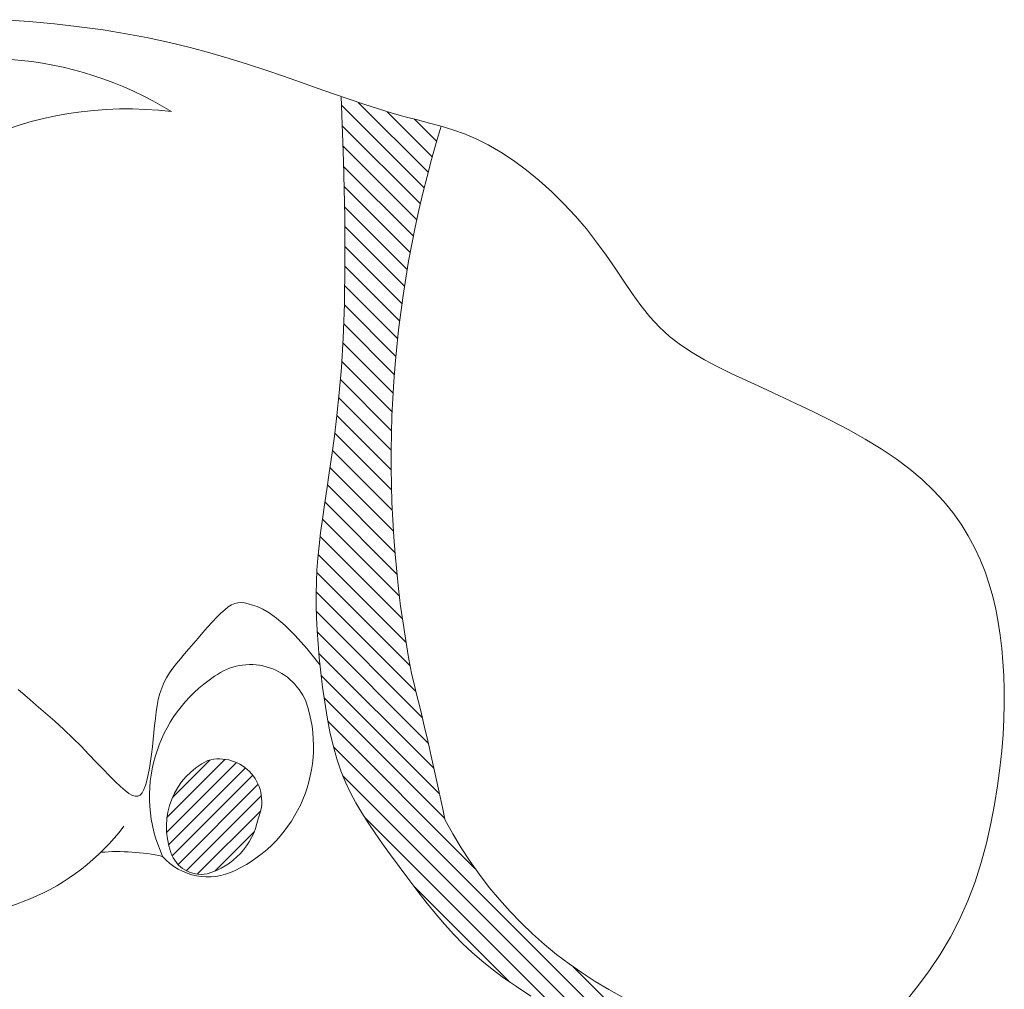
# Model space of a CAD drawing. Units: inches. Extents: x -17 to 1735, y -531 to 60.
# Tile 9 of 27: x 1734.675388 to 1734.678793, y -150.220021 to -150.216668. Entities that reach past the tile are written whole.
import ezdxf

# ---------------------------------------------------------------- set-up
doc = ezdxf.new("R2010")
doc.units = ezdxf.units.IN
doc.header["$MEASUREMENT"] = 0
doc.layers.add('A-FURN', color=242, linetype='Continuous', lineweight=18, true_color=0xcd2027)

# ---------------------------------------------------------------- blocks, each defined once
blk = doc.blocks.new('childrens_room_2')
for p, q in [((70.17339440191746, 54.15018009333147), (70.17563597329311, 54.15001020629865)), ((70.17563597329311, 54.15001020629865), (70.17785059184419, 54.14980570076153)), ((70.17785059184419, 54.14980570076153), (70.18001900573611, 54.14956273020511)), ((70.18001900573611, 54.14956273020511), (70.18212196290145, 54.14927744811433)), ((70.18212196290145, 54.14927744811433), (70.18414438255016, 54.14894745044733)), ((70.18414438255016, 54.14894745044733), (70.18608786917642, 54.14857610287294)), ((70.18608786917642, 54.14857610287294), (70.18795819820255, 54.14816821353309)), ((70.18795819820255, 54.14816821353309), (70.18976114540013, 54.14772859055523)), ((70.18976114540013, 54.14772859055523), (70.19150248619147, 54.14726204206676)), ((70.19150248619147, 54.14726204206676), (70.19318799628994, 54.14677337620964)), ((70.19318799628994, 54.14677337620964), (70.19482345123427, 54.14626740109674)), ((70.19482345123427, 54.14626740109674), (70.19641462662142, 54.14574892487729)), ((70.19641462662142, 54.14574892487729), (70.1979658542073, 54.14522323648128)), ((70.1979658542073, 54.14522323648128), (70.19947568997625, 54.14469754809255)), ((70.19947568997625, 54.14469754809255), (70.20094124624623, 54.14417955271932)), ((70.20094124624623, 54.14417955271932), (70.20235963521876, 54.14367694335528)), ((70.20235963521876, 54.14367694335528), (70.20372796909535, 54.14319741299408)), ((70.20304380218616, 54.14343717817832), (70.20324643027155, 54.13775630528693)), ((70.21032588458505, 54.13540639450224), (70.2030714949465, 54.14266078414079)), ((70.20372796909535, 54.14319741299408), (70.20504336001935, 54.14274865464398)), ((70.21067641210858, 54.13678467516587), (70.20454107237632, 54.14292001493453)), ((70.20504336001935, 54.14274865464398), (70.20630292025047, 54.14233836128409)), ((70.20630292025047, 54.14233836128409), (70.20750376199024, 54.14197422592991)), ((70.21104344307562, 54.13814645241513), (70.20709029149614, 54.14209960400916)), ((70.20750376199024, 54.14197422592991), (70.20864556439804, 54.14165913344771)), ((70.20864556439804, 54.14165913344771), (70.20973827429, 54.14137673621593)), ((70.21142657864723, 54.13949212503069), (70.20947355376441, 54.14144514992807)), ((70.20973827429, 54.14137673621593), (70.21079440544011, 54.14110587847102)), ((70.21079440544011, 54.14110587847102), (70.21182647162235, 54.14082540447856)), ((70.20999228646863, 54.13401118443147), (70.2031354397291, 54.14086803115646)), ((70.21182544513024, 54.14082206677125), (70.21182047879441, 54.14082703307798)), ((70.21182647162235, 54.14082540447856), (70.21284698661069, 54.14051415846774)), ((70.21284698661069, 54.14051415846774), (70.21386846423732, 54.14015098470412)), ((70.21386846423732, 54.14015098470412), (70.21490341821801, 54.13971472742417)), ((70.21490341821801, 54.13971472742417), (70.21596436232679, 54.1391842308862)), ((70.21596436232679, 54.1391842308862), (70.21705931827776, 54.13854378854598)), ((70.20967607329251, 54.13259858941313), (70.20319938451169, 54.13907527817213)), ((70.21705931827776, 54.13854378854598), (70.2181783391384, 54.13779949069288)), ((70.20324643027155, 54.13775630528693), (70.20335176733673, 54.13288732946097)), ((70.2181783391384, 54.13779949069288), (70.21930698597455, 54.13696287682836)), ((70.20937773283688, 54.13116812163792), (70.20325653320063, 54.13728932131784)), ((70.21930698597455, 54.13696287682836), (70.22043081979385, 54.13604548646111)), ((70.22043081979385, 54.13604548646111), (70.22153540166212, 54.13505885909256)), ((70.2090977882722, 54.1297192580518), (70.20329476183863, 54.13552228446355)), ((70.22153540166212, 54.13505885909256), (70.22260629252881, 54.13401453422415)), ((70.22260629252881, 54.13401453422415), (70.22362905351795, 54.13292405136457)), ((70.20883680112777, 54.12825143695812), (70.20333299053485, 54.13375524760198)), ((70.20335176733673, 54.13288732946097), (70.20337261184935, 54.12873569591323)), ((70.22362905351795, 54.13292405136457), (70.22458924563719, 54.13179895001525)), ((70.20859537571553, 54.12676405418318), (70.20335620625295, 54.13200322366032)), ((70.22458924563719, 54.13179895001525), (70.22547772411374, 54.13065125048018)), ((70.22547772411374, 54.13065125048018), (70.22630652157707, 54.12949489633177)), ((70.20837416302994, 54.1252564587034), (70.20336493006792, 54.13026569165089)), ((70.22630652157707, 54.12949489633177), (70.22709296464339, 54.128344311945)), ((70.20337261184935, 54.12873569591323), (70.20332176250989, 54.12520684984196)), ((70.20817386581214, 54.12372794771221), (70.20336967864888, 54.12853213488273)), ((70.22709296464339, 54.128344311945), (70.22785438016174, 54.12721392168027)), ((70.22785438016174, 54.12721392168027), (70.22860809492298, 54.12611814991254)), ((70.20799524442876, 54.12217776090114), (70.20334512101138, 54.12682788428941)), ((70.22860809492298, 54.12611814991254), (70.22937143560151, 54.12507142102407)), ((70.20332176250989, 54.12520684984196), (70.20321201796062, 54.12220623646721)), ((70.2078391231585, 54.12060507396967), (70.20331878408209, 54.12512541304607)), ((70.22937143560151, 54.12507142102407), (70.23016172904639, 54.12408815938255)), ((70.23016172904639, 54.12408815938255), (70.23099630204845, 54.12318278935567)), ((70.20770639787546, 54.11900899106552), (70.20325778553845, 54.12345760340253)), ((70.23099630204845, 54.12318278935567), (70.23188991438249, 54.12236460665593)), ((70.20321201796062, 54.12220623646721), (70.20305617678562, 54.11963930099449)), ((70.23188991438249, 54.12236460665593), (70.23284705816653, 54.12162239232424)), ((70.20759804466391, 54.11738853608989), (70.203187310613, 54.12179927008986)), ((70.23284705816653, 54.12162239232424), (70.23386965867715, 54.12093979873174)), ((70.20751513006283, 54.11574264248923), (70.20308836032521, 54.1201694121832)), ((70.23386965867715, 54.12093979873174), (70.23495964107452, 54.12030047826414)), ((70.23495964107452, 54.12030047826414), (70.23611893057708, 54.1196880832926)), ((70.20305617678562, 54.11963930099449), (70.20286703756895, 54.11741148862205)), ((70.23611893057708, 54.1196880832926), (70.23734945240315, 54.11908626620283)), ((70.20745882294025, 54.1140701413737), (70.20296489093337, 54.11856407339513)), ((70.23734945240315, 54.11908626620283), (70.23865313171294, 54.1184786793587)), ((70.23865313171294, 54.1184786793587), (70.24003189378303, 54.11784897514593)), ((70.24003189378303, 54.11784897514593), (70.24148333207587, 54.11718385109129)), ((70.20286703756895, 54.11741148862205), (70.20265739895288, 54.11542824456268)), ((70.20743040869596, 54.11236974745264), (70.20282130561421, 54.11697885053439)), ((70.24148333207587, 54.11718385109129), (70.24298771332136, 54.11648218528575)), ((70.24298771332136, 54.11648218528575), (70.24452097255156, 54.11574590099775)), ((70.20265739895288, 54.11542824456268), (70.20243872866152, 54.1136086095052)), ((70.2074313055596, 54.11064004237999), (70.20265586535564, 54.11541548261306)), ((70.24452097255156, 54.11574590099775), (70.2460590447404, 54.11497692145935)), ((70.2460590447404, 54.11497692145935), (70.24757786497824, 54.11417716993168)), ((70.24757786497824, 54.11417716993168), (70.24905336829718, 54.11334856966863)), ((70.20243872866152, 54.1136086095052), (70.2022171706299, 54.11192600602811)), ((70.20746308484698, 54.10887945489815), (70.20247039805282, 54.11387214171412)), ((70.24905336829718, 54.11334856966863), (70.25046148967115, 54.11249304390953)), ((70.20752749465056, 54.1070862369001), (70.2022719218617, 54.11234180968171)), ((70.25046148967115, 54.11249304390953), (70.25177816413228, 54.11161251591551)), ((70.2022171706299, 54.11192600602811), (70.20199753775844, 54.1103674521932)), ((70.25177816413228, 54.11161251591551), (70.25298430014983, 54.11070874865839)), ((70.20762648888515, 54.10525843444196), (70.20206175733941, 54.11082316598771)), ((70.25298430014983, 54.11070874865839), (70.25408069988364, 54.10978286403263)), ((70.20199753775844, 54.1103674521932), (70.20178464306403, 54.10891996606228)), ((70.25408069988364, 54.10978286403263), (70.25507313898882, 54.1088358236579)), ((70.20178464306403, 54.10891996606228), (70.20158329962172, 54.10757056568257)), ((70.20776226285263, 54.1033938522873), (70.20184253535584, 54.1093135797841)), ((70.25507313898882, 54.1088358236579), (70.2559673929459, 54.10786858916111)), ((70.20158329962172, 54.10757056568257), (70.20139832033195, 54.10630626912319)), ((70.20793729683967, 54.10149001013491), (70.20161880239496, 54.10780850456507)), ((70.2559673929459, 54.10786858916111), (70.25676923746826, 54.10688212215467)), ((70.20139832033195, 54.10630626912319), (70.20123451821158, 54.10511409444592)), ((70.2081544108328, 54.09954408793277), (70.20139758458711, 54.10630091417846)), ((70.25676923746826, 54.10688212215467), (70.25748444815284, 54.10587738426551)), ((70.25748444815284, 54.10587738426551), (70.25811880059658, 54.10485533711329)), ((70.20123451821158, 54.10511409444592), (70.20109670621926, 54.10398105969801)), ((70.20841683361098, 54.09755285692376), (70.20119342750289, 54.10477626306096)), ((70.25811880059658, 54.10485533711329), (70.25867807028001, 54.10381694232495)), ((70.20109670621926, 54.10398105969801), (70.20098873479176, 54.10289394254363)), ((70.25867807028001, 54.10381694232495), (70.25916787255439, 54.10276300123809)), ((70.20098873479176, 54.10289394254363), (70.20091060392909, 54.10183855901272)), ((70.20872829098838, 54.09551259138829), (70.2010210972035, 54.10321978516589)), ((70.25916787255439, 54.10276300123809), (70.2595931807405, 54.10169367413477)), ((70.20091060392909, 54.10183855901272), (70.20086135099294, 54.10080048472304)), ((70.209093120076, 54.09341895411348), (70.20089986444103, 54.10161220969752)), ((70.2595931807405, 54.10169367413477), (70.25995880779695, 54.10060896102226)), ((70.20086135099294, 54.10080048472304), (70.20084001340322, 54.09976529530689)), ((70.25995880779695, 54.10060896102226), (70.26026956679883, 54.09950886190057)), ((70.20084001340322, 54.09976529530689), (70.20084562857986, 54.09871856638204)), ((70.20960674738629, 54.09117651853597), (70.20084360743525, 54.09993965853795)), ((70.26026956679883, 54.09950886190057), (70.26053027064657, 54.09839337677698)), ((70.19311731239898, 54.09859969038956), (70.19280515798484, 54.09835607694407)), ((70.19340699982016, 54.09877877666298), (70.19311731239898, 54.09859969038956)), ((70.19368443254965, 54.09889818168307), (70.19340699982016, 54.09877877666298)), ((70.19395982288873, 54.09896275136128), (70.19368443254965, 54.09889818168307)), ((70.19424338302227, 54.09897733160182), (70.19395982288873, 54.09896275136128)), ((70.19454532525154, 54.09894676833068), (70.19424338302227, 54.09897733160182)), ((70.19487586187782, 54.09887590745205), (70.19454532525154, 54.09894676833068)), ((70.19524520496955, 54.09876959488468), (70.19487586187782, 54.09887590745205)), ((70.19566427218845, 54.0986253894211), (70.19524520496955, 54.09876959488468)), ((70.1961468013574, 54.098411701349), (70.19566427218845, 54.0986253894211)), ((70.20084562857986, 54.09871856638204), (70.20087723388454, 54.09764587358807)), ((70.19209438557621, 54.09767798904653), (70.19170529896977, 54.09726421601084)), ((70.19246304769652, 54.09804585343085), (70.19209438557621, 54.09767798904653)), ((70.19280515798484, 54.09835607694407), (70.19246304769652, 54.09804585343085)), ((70.19670723589255, 54.09808965385167), (70.1961468013574, 54.098411701349)), ((70.19736001891899, 54.0976203700979), (70.19670723589255, 54.09808965385167)), ((70.21016131819809, 54.08889313957337), (70.20086110314472, 54.09819335459764)), ((70.20087723388454, 54.09764587358807), (70.2009338667954, 54.09653279253546)), ((70.26053027064657, 54.09839337677698), (70.26074573235702, 54.09726250565149)), ((70.19130191522302, 54.09681626652894), (70.19089036162362, 54.09634587282056)), ((70.19170529896977, 54.09726421601084), (70.19130191522302, 54.09681626652894)), ((70.19811959367829, 54.09696497326371), (70.19736001891899, 54.0976203700979)), ((70.19900040341193, 54.09608458652513), (70.19811959367829, 54.09696497326371)), ((70.26074573235702, 54.09726250565149), (70.2609207650053, 54.09611624853136)), ((70.19089036162362, 54.09634587282056), (70.1904767655756, 54.09586476709086)), ((70.20001689130324, 54.09494033305822), (70.19900040341193, 54.09608458652513)), ((70.2009338667954, 54.09653279253546), (70.20101456461592, 54.09536489886381)), ((70.21069031529944, 54.08663533424117), (70.20094433328953, 54.0963813162511)), ((70.2609207650053, 54.09611624853136), (70.26106018143358, 54.0949546054166)), ((70.1900672544248, 54.09538468155955), (70.18966795551708, 54.09491734843908)), ((70.1904767655756, 54.09586476709086), (70.1900672544248, 54.09538468155955)), ((70.20101456461592, 54.09536489886381), (70.20111884608517, 54.09413353793064)), ((70.18928440044286, 54.09447143936853), (70.18891973806197, 54.09404338367171)), ((70.18966795551708, 54.09491734843908), (70.18928440044286, 54.09447143936853)), ((70.20118350065198, 54.09349333603171), (70.20001689130324, 54.09494033305822)), ((70.2111947168701, 54.08440212451973), (70.20108697564459, 54.09450986570885)), ((70.26106018143358, 54.0949546054166), (70.26116767165834, 54.09377629415252)), ((70.18857652136242, 54.09362655009903), (70.18825730339043, 54.09321430740096)), ((70.18891973806197, 54.09404338367171), (70.18857652136242, 54.09362655009903)), ((70.20111884608517, 54.09413353793064), (70.20124815516058, 54.09285313413278)), ((70.26116767165834, 54.09377629415252), (70.26124243351981, 54.09257490389285)), ((70.18796463730862, 54.09280002432064), (70.1877010760468, 54.09237706960851)), ((70.18825730339043, 54.09321430740096), (70.18796463730862, 54.09280002432064)), ((70.20124815516058, 54.09285313413278), (70.20140441700235, 54.0915438815777)), ((70.21167543554795, 54.08219259764013), (70.20127976774123, 54.0925882654032)), ((70.26124243351981, 54.09257490389285), (70.2612825417996, 54.09134274163665)), ((70.18746917282581, 54.09193881202231), (70.18727148057545, 54.09147862030517)), ((70.1877010760468, 54.09237706960851), (70.18746917282581, 54.09193881202231)), ((70.17544705514914, 54.09067334845025), (70.17466624338297, 54.09133766362941)), ((70.18710919074832, 54.09099130847465), (70.1869780483062, 54.09047747165317)), ((70.18727148057545, 54.09147862030517), (70.18710919074832, 54.09099130847465)), ((70.20140441700235, 54.0915438815777), (70.20158955677064, 54.09022597440202)), ((70.2612825417996, 54.09134274163665), (70.26128607139574, 54.09007211438296)), ((70.17625441880548, 54.08998454865508), (70.17544705514914, 54.09067334845025)), ((70.17707352649771, 54.08927636522133), (70.17625441880548, 54.08998454865508)), ((70.18687243650086, 54.08993915021568), (70.18678673858406, 54.0893783845517)), ((70.1869780483062, 54.09047747165317), (70.18687243650086, 54.08993915021568)), ((70.21213332489017, 54.08000590009618), (70.20153665217688, 54.09060257278764)), ((70.20158955677064, 54.09022597440202), (70.20180549974205, 54.08891960672775)), ((70.26128607139574, 54.09007211438296), (70.26125109697344, 54.08875532912356)), ((70.17788957054611, 54.08855389910462), (70.17707352649771, 54.08927636522133)), ((70.18678673858406, 54.0893783845517), (70.18671533780756, 54.08879721503621)), ((70.17868774315458, 54.08782225126782), (70.17788957054611, 54.08855389910462)), ((70.1866526174231, 54.08819768207326), (70.18659296079889, 54.08758182603782)), ((70.18671533780756, 54.08879721503621), (70.1866526174231, 54.08819768207326)), ((70.20180549974205, 54.08891960672775), (70.20205417101855, 54.08764497268425)), ((70.21479319339736, 54.07561722337999), (70.20188177372214, 54.08852864305521)), ((70.26125109697344, 54.08875532912356), (70.26117569343072, 54.08738469285748)), ((70.17945519387607, 54.08708762787722), (70.17868774315458, 54.08782225126782)), ((70.18659296079889, 54.08758182603782), (70.18653075112846, 54.08695168730486)), ((70.20205417101855, 54.08764497268425), (70.20233749587672, 54.0864222664008)), ((70.26117569343072, 54.08738469285748), (70.26105793554918, 54.08595251258379)), ((70.18018690171769, 54.08636065594186), (70.17945519387607, 54.08708762787722)), ((70.18653075112846, 54.08695168730486), (70.18646122271778, 54.08631109160928)), ((70.20233749587672, 54.0864222664008), (70.20265739941854, 54.0852716819922)), ((70.18087980291924, 54.08565306766689), (70.18018690171769, 54.08636065594186)), ((70.1815308339533, 54.08497659525022), (70.18087980291924, 54.08565306766689)), ((70.18638301391503, 54.08567100601652), (70.18629561412266, 54.08504418291562)), ((70.18646122271778, 54.08631109160928), (70.18638301391503, 54.08567100601652)), ((70.23120320653427, 54.05747840204134), (70.20236759360299, 54.08631401495807)), ((70.26105793554918, 54.08595251258379), (70.26089589816868, 54.08445109528696)), ((70.18213693111785, 54.08434297091156), (70.1815308339533, 54.08497659525022)), ((70.18629561412266, 54.08504418291562), (70.1861985126848, 54.08444337472468)), ((70.18770175247803, 54.07879595101843), (70.19384133135785, 54.08493552992007)), ((70.187735999421, 54.0801029901981), (70.19285216655001, 54.08521915729801)), ((70.18821561488906, 54.08185539782284), (70.19153095759569, 54.08517074053674)), ((70.20265739941854, 54.0852716819922), (70.20301564655848, 54.08420700275605)), ((70.18269503059449, 54.0837639268488), (70.18213693111785, 54.08434297091156)), ((70.18609119906208, 54.08388133384), (70.18597316254048, 54.0833708126724)), ((70.1861985126848, 54.08444337472468), (70.18609119906208, 54.08388133384)), ((70.1878786482371, 54.07770005457718), (70.19463595888693, 54.08445736520519)), ((70.18819652929554, 54.07674514342073), (70.19527148875525, 54.0838201029241)), ((70.20301564655848, 54.08420700275605), (70.20341336018058, 54.08321636865588)), ((70.26089589816868, 54.08445109528696), (70.26068685385283, 54.08287691501612)), ((70.18320206885576, 54.08325119527439), (70.18269503059449, 54.0837639268488)), ((70.18365498219967, 54.08281650839348), (70.18320206885576, 54.08325119527439)), ((70.18597316254048, 54.0833708126724), (70.1858438925806, 54.0829245636109)), ((70.18870862795623, 54.07598444991021), (70.1957477533247, 54.08302357525684)), ((70.22698188498501, 54.05997091540342), (70.20319665329183, 54.0837561470675)), ((70.20341336018058, 54.08321636865588), (70.20385150298128, 54.08228150880171)), ((70.18405215361739, 54.08246964304857), (70.18365498219967, 54.08281650839348)), ((70.18439775322216, 54.08221255460961), (70.18405215361739, 54.08246964304857)), ((70.1846973976458, 54.0820452430766), (70.18439775322216, 54.08221255460961)), ((70.18537676748704, 54.08208196992785), (70.18518128805911, 54.08197995072845)), ((70.18554875872681, 54.08227376604049), (70.18537676748704, 54.08208196992785)), ((70.18570287852666, 54.08255533906634), (70.18554875872681, 54.08227376604049)), ((70.1858438925806, 54.0829245636109), (70.18570287852666, 54.08255533906634)), ((70.20385150298128, 54.08228150880171), (70.20433103754068, 54.08138415233264)), ((70.26068685385283, 54.08287691501612), (70.26042486664258, 54.08124311397699)), ((70.18495670369478, 54.08196770844956), (70.1846973976458, 54.0820452430766)), ((70.18518128805911, 54.08197995072845), (70.18495670369478, 54.08196770844956)), ((70.18943195046043, 54.07543498018497), (70.19602876297316, 54.08203179271225)), ((70.20433103754068, 54.08138415233264), (70.20485292643892, 54.08050602835141)), ((70.26042486664258, 54.08124311397699), (70.26010319830269, 54.07956700143262)), ((70.19040159847239, 54.07513183601117), (70.19597454946373, 54.0807047870025)), ((70.20485292643892, 54.08050602835141), (70.20541813225603, 54.07962886598983)), ((70.22263468104532, 54.06258931114138), (70.2050974529225, 54.08012653924237)), ((70.20541813225603, 54.07962886598983), (70.20602761757212, 54.0787343943652)), ((70.26010319830269, 54.07956700143262), (70.25971511065612, 54.07786588663151)), ((70.19193352701726, 54.07539097236298), (70.19540032256512, 54.07885776788901)), ((70.20602761757212, 54.0787343943652), (70.20668234502548, 54.07780434260934)), ((70.20668234502548, 54.07780434260934), (70.20738183335519, 54.07682620959389)), ((70.25971511065612, 54.07786588663151), (70.25925386552584, 54.07615707882218)), ((70.20738183335519, 54.07682620959389), (70.20811982558692, 54.07581057318606)), ((70.25925386552584, 54.07615707882218), (70.2587127247348, 54.07445788726767)), ((70.20811982558692, 54.07581057318606), (70.20888862096356, 54.07477378102925)), ((70.20888862096356, 54.07477378102925), (70.20968051872799, 54.07373218073775)), ((70.2587127247348, 54.07445788726767), (70.25808495004777, 54.0727856212165)), ((70.217824109433, 54.0656710745447), (70.20941893035663, 54.07407625362106)), ((70.20968051872799, 54.07373218073775), (70.21048781806488, 54.07270211995495)), ((70.21048781806488, 54.07270211995495), (70.21130281815888, 54.07169994630243)), ((70.25808495004777, 54.0727856212165), (70.25736380328775, 54.07115758993171)), ((70.21130281815888, 54.07169994630243), (70.21211781825289, 54.0707420074163)), ((70.25736380328775, 54.07115758993171), (70.25654655707652, 54.0695885383306)), ((70.21211781825289, 54.0707420074163), (70.21292511758978, 54.06984465091813)), ((70.21292511758978, 54.06984465091813), (70.21372280393146, 54.06901777622846)), ((70.25654655707652, 54.0695885383306), (70.25564652740607, 54.06808295399099)), ((70.21372280393146, 54.06901777622846), (70.21453211987274, 54.06824548994194)), ((70.21453211987274, 54.06824548994194), (70.21538009658573, 54.06750545043036)), ((70.21538009658573, 54.06750545043036), (70.21629376518425, 54.0667753160655)), ((70.25564652740607, 54.06808295399099), (70.25468104100904, 54.06664276016676)), ((70.21629376518425, 54.0667753160655), (70.21730015684037, 54.06603274524099)), ((70.23229530256825, 54.0581151142091), (70.22340834805394, 54.06700206872341)), ((70.25468104100904, 54.06664276016676), (70.25366742467625, 54.06526988009722)), ((70.21730015684037, 54.06603274524099), (70.21842630278437, 54.06525539631406)), ((70.21842630278437, 54.06525539631406), (70.2196992340719, 54.06442092767832)), ((70.25366742467625, 54.06526988009722), (70.25262300519854, 54.06396623705081))]:
    blk.add_line(p, q)
for centre, radius, start, end in [((70.17166475667503, 54.11546908731401), 0.0313149888669701, 58.27266326727306, 113.0496076004186), ((70.18419688196039, 54.11024985505941), 0.0320967331381597, 82.95662561159509, 211.3772048657365), ((70.30698901503231, 54.11155651698795), 0.0995619276835286, 162.9038136953596, 190.9501850460958), ((70.19505898253877, 54.08824078469336), 0.0052968842846864, 23.09790550296972, 126.3443002049826), ((70.19879745145911, 54.08195893498344), 0.0125924033173701, 123.1046590961696, 204.71759410843), ((69.93031475443743, 54.02213504049581), 0.2876990494333318, 11.58866688267244, 14.18653306617982), ((70.18856446224848, 54.08633654655426), 0.0120441644060298, 295.3327286808845, 19.30733223293256), ((70.19418402255863, 54.07928007116282), 0.0065003228993452, 116.0081285668524, 200.1726280298054), ((70.19232629054343, 54.08151844328535), 0.0037378910829727, 335.9921885959464, 105.4004929466278), ((70.16805124132544, 54.09132497389368), 0.0199068323432125, 201.8074763810449, 322.9514703004661), ((70.18957163429471, 54.08121966064067), 0.0062890495654325, 285.5858718760119, 348.7956284868045), ((70.2447362221533, 54.09694509747208), 0.0367622521574525, 207.5719883014331, 277.4112487822124), ((70.1834215496888, 54.05836710254374), 0.018744531838257, 77.87494330126607, 94.57002885024384), ((70.19073528034961, 54.07790151097145), 0.0027897030266892, 198.021797321194, 280.8705143621302), ((70.191338051121, 54.08016376169547), 0.0052799262236599, 221.0913232052541, 296.7902562470012)]:
    blk.add_arc(centre, radius, start, end)

msp = doc.modelspace()

# ---------------------------------------------------------------- block references
at = {"layer": 'A-FURN', "xscale": 0.0393700787401575, "yscale": 0.0393700787401575, "zscale": 0.0393700787401575}
msp.add_blockref('childrens_room_2', (1731.912600860487, -152.3485650223338), dxfattribs=at)

doc.saveas('drawing.dxf')
